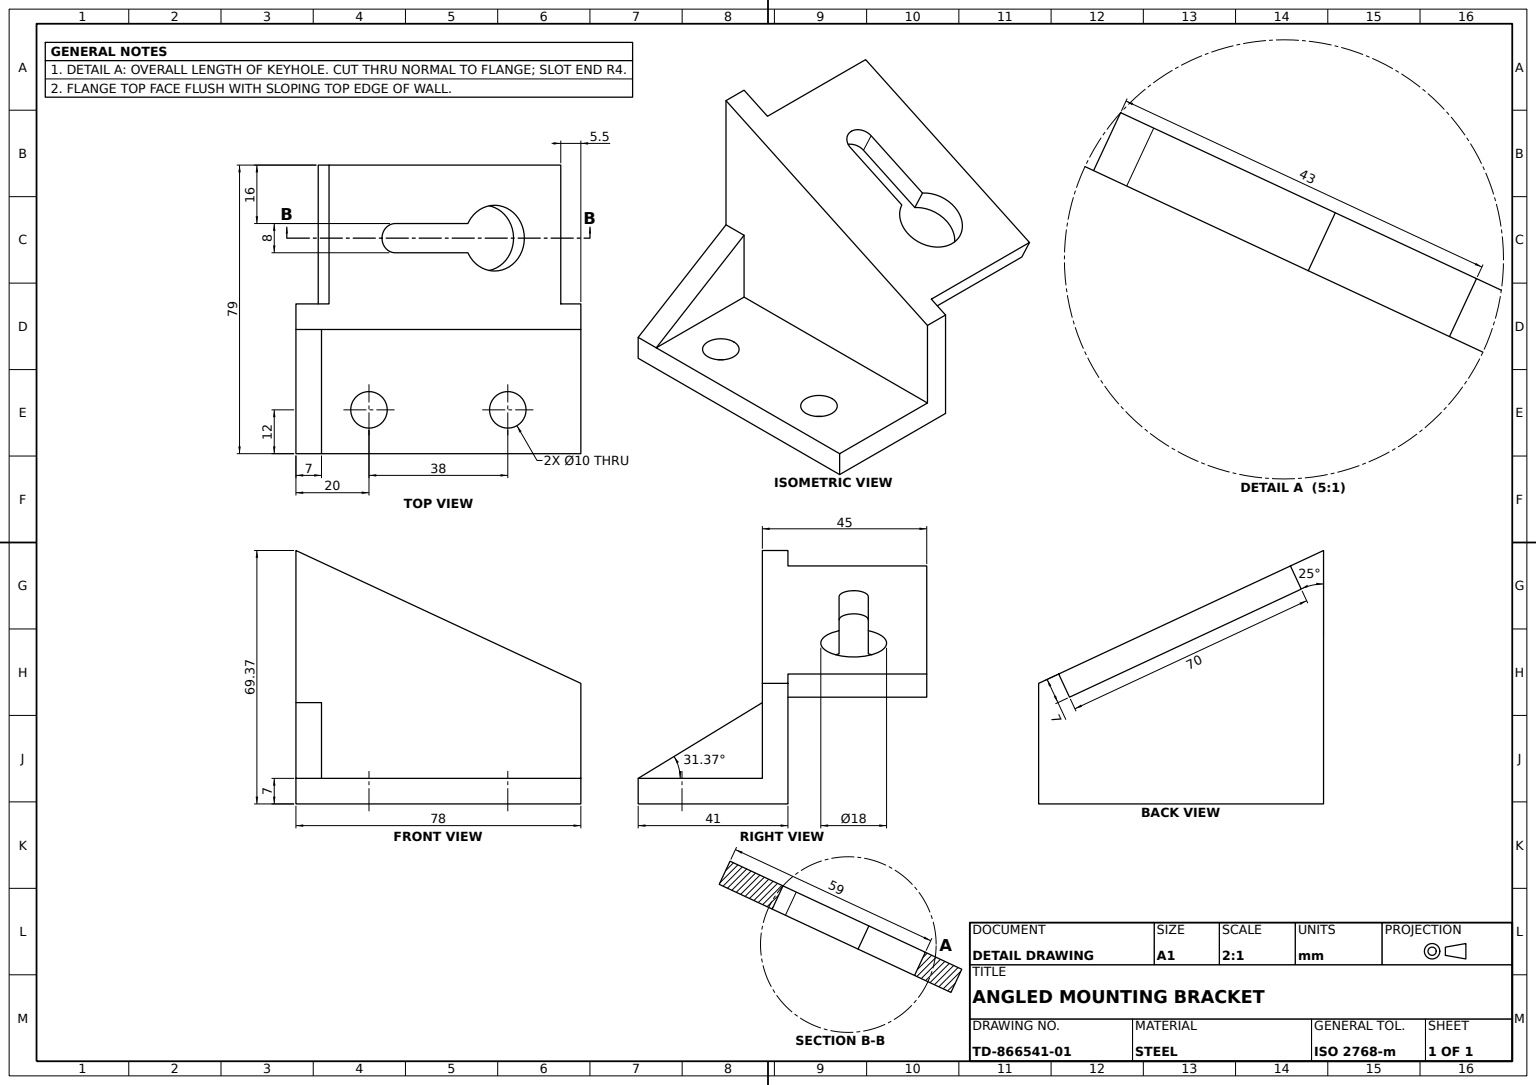
SolidWorks part; units mm, degrees
material "Plain Carbon Steel"
ref_plane "Front Plane" through (0, 0, 0) normal (0, 0, 1) x (1, 0, 0)
ref_plane "Top Plane" through (0, 0, 0) normal (0, 1, 0) x (1, 0, 0)
ref_plane "Right Plane" through (0, 0, 0) normal (1, 0, 0) x (0, 0, -1)
sketch "Base Plate Sketch" plane through (0, 0, 0) normal (0, 1, 0) x (1, 0, 0)
  line L1 (-39, 20.5) -> (39, 20.5)
  line L2 (-39, 20.5) -> (-39, -20.5)
  line L3 (-39, -20.5) -> (39, -20.5)
  line L4 (39, 20.5) -> (39, -20.5)
  line L5 (-39, 20.5) -> (39, -20.5) construction
  line L6 (-39, -20.5) -> (39, 20.5) construction
  circle A0 centre (-19, -8.5) radius 5
  circle A1 centre (19, -8.5) radius 5
  point P0 (0, 0)
  dimension "D3" = 10
  dimension "D1" = 78
  dimension "D2" = 41
  dimension "D4" = 20
  dimension "D5" = 20
  dimension "D6" = 12
extrude "Base Plate" add sketch "Base Plate Sketch" along normal blind 7
sketch "Gusset Sketch" plane through (-39, 0, 0) normal (-1, 0, 0) x (0, 0, 1)
  line L0 (-20.5, 7) -> (-20.5, 32)
  line L1 (-20.5, 7) -> (20.5, 7)
  line L2 (20.5, 7) -> (-20.5, 32)
  dimension "D1" = 25
  dimension "D2" = 41
extrude "Gusset" add sketch "Gusset Sketch" against normal blind 7
sketch "Upright Wall Sketch" plane through (0, 0, -20.5) normal (0, 0, -1) x (-1, 0, 0)
  line L0 (-39, 7) -> (-39, 33)
  line L1 (-39, 33) -> (39, 69.372)
  line L2 (39, 69.372) -> (39, 7)
  line L3 (39, 32) -> (39, 0) construction
  line L4 (39, 7) -> (-39, 7)
  line L5 (-39, 0) -> (39, 0) construction
  dimension "D1" = 25
  dimension "D2" = 33
extrude "Upright Wall" add sketch "Upright Wall Sketch" against normal blind 7
ref_plane "Flange Plane" through (19.6054, 42.0439, 0) normal (0.4226, 0.9063, 0) x (0.9063, -0.4226, 0)
sketch "Keyhole Flange Sketch" plane through (19.6054, 42.0439, 0) normal (0.4226, 0.9063, 0) x (0.9063, -0.4226, 0)
  line L0 (-64.6639, 20.5) -> (21.3996, 20.5) construction
  line L1 (-54.6639, 20.5) -> (15.3361, 20.5)
  line L2 (-54.6639, 20.5) -> (-54.6639, 58.5)
  line L3 (-54.6639, 58.5) -> (15.3361, 58.5)
  line L4 (15.3361, 20.5) -> (15.3361, 58.5)
  line L5 (-64.6639, 13.5) -> (21.3996, 13.5) construction
  line L6 (-64.6639, 13.5) -> (-64.6639, 20.5) construction
  line L7 (-34.6639, 38.5) -> (-4.6639, 38.5) construction
  line L8 (-34.6639, 42.5) -> (-12.7261, 42.5)
  line L9 (-34.6639, 34.5) -> (-12.7261, 34.5)
  arc A0 (-34.6639, 42.5) -> (-34.6639, 34.5) centre (-34.6639, 38.5) ccw
  arc A2 (-12.7261, 34.5) -> (-12.7261, 42.5) centre (-4.6639, 38.5) ccw
  point P12 (-19.6639, 38.5)
  point P20 (-19.6639, 58.5)
  dimension "D6" = 20
  dimension "D7" = 18
  dimension "D1" = 45
  dimension "D2" = 10
  dimension "D3" = 70
  dimension "D4" = 8
  dimension "D5" = 20
extrude "Keyhole Mounting Flange" add sketch "Keyhole Flange Sketch" against normal blind 7
